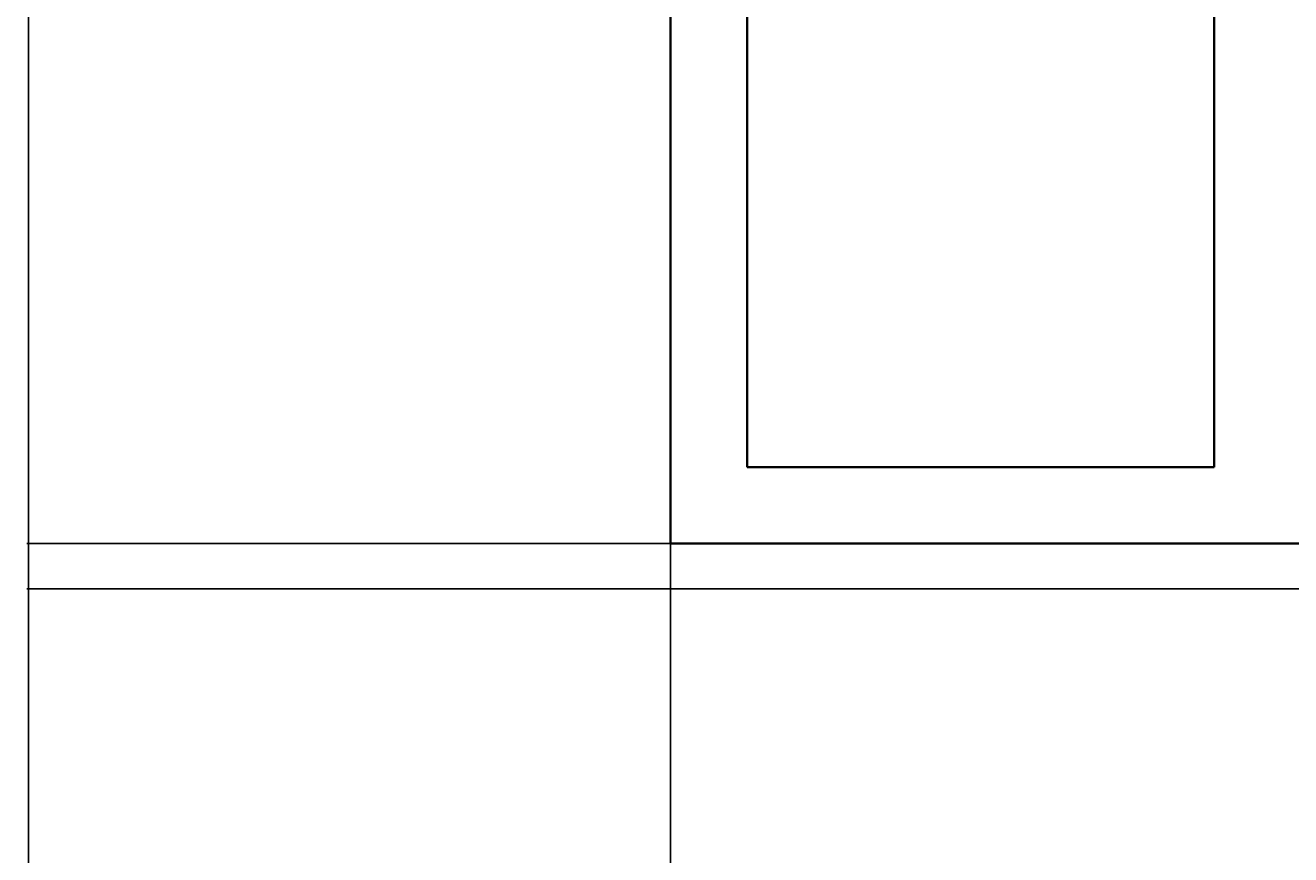
# Model space of a CAD drawing. Units: inches. Extents: x -61 to 1599, y -1316 to 257.
# Tile 43 of 204: x -61 to 88, y -478 to -380. Entities that reach past the tile are written whole.
import ezdxf

# ---------------------------------------------------------------- set-up
doc = ezdxf.new("R2010")
doc.units = ezdxf.units.IN
doc.header["$MEASUREMENT"] = 0
doc.layers.add('A-ANNO-DIMS', color=2, linetype='Continuous', lineweight=18)
doc.layers.add('WALLS', color=4, linetype='Continuous', lineweight=35)
doc.styles.get("Standard").update_dxf_attribs({"font": 'arial.ttf'})
doc.dimstyles.get("Standard").update_dxf_attribs({"dimtxt": 0.18, "dimasz": 0.18, "dimexe": 0.18, "dimexo": 0.0625, "dimgap": 0.09, "dimtad": 0, "dimtih": 1, "dimtoh": 1, "dimdec": 0, "dimzin": 0, "dimdsep": 46, "dimlunit": 3, "dimtxsty": 'Standard', "dimcen": 0.09, "dimadec": 0, "dimazin": 0, "dimtfac": 1, "dimtdec": 0, "dimtofl": 0, "dimtmove": 0, "dimatfit": 3, "dimfxl": 1, "dimtolj": 1, "dimtzin": 0, "dimarcsym": 0})

# ---------------------------------------------------------------- blocks, each defined once
blk = doc.blocks.new('*D687')
at = {"layer": 'A-ANNO-DIMS', "color": 0, "lineweight": -2, "transparency": 16777216}
for p, q in [((289.42, 181.68), (-61.08, 181.68)), ((-60.9, 181.5), (-60.9, -528.95)), ((-60.9, -1239.76), (-60.9, -529.32)), ((319.64, -1239.94), (-61.08, -1239.94))]:
    blk.add_line(p, q, dxfattribs=at)
at = {"layer": 'A-ANNO-DIMS', "color": 0, "transparency": 16777216}
for points in [[(-60.93, 181.5), (-60.87, 181.5), (-60.9, 181.68)], [(-60.93, -1239.76), (-60.87, -1239.76), (-60.9, -1239.94)]]:
    blk.add_solid(points, dxfattribs=at)
at = {"layer": 'DEFPOINTS', "color": 0, "transparency": 16777216}
for p in [(289.48, 181.68), (-60.9, -1239.94), (319.7, -1239.94)]:
    blk.add_point(p, dxfattribs=at)
at = {"layer": 'A-ANNO-DIMS', "color": 0, "transparency": 16777216, "insert": (-60.9, -529.13), "char_height": 0.18, "attachment_point": 5}
blk.add_mtext('\\A1;1421.6', dxfattribs=at)
blk = doc.blocks.new('*D691')
at = {"layer": 'A-ANNO-DIMS', "color": 0, "lineweight": -2, "transparency": 16777216}
for p, q in [((14.64, 157.68), (-61.08, 157.68)), ((-60.9, 157.5), (-60.9, -141.64)), ((-60.9, -441.14), (-60.9, -142)), ((14.64, -441.32), (-61.08, -441.32))]:
    blk.add_line(p, q, dxfattribs=at)
at = {"layer": 'A-ANNO-DIMS', "color": 0, "transparency": 16777216}
for points in [[(-60.93, 157.5), (-60.87, 157.5), (-60.9, 157.68)], [(-60.93, -441.14), (-60.87, -441.14), (-60.9, -441.32)]]:
    blk.add_solid(points, dxfattribs=at)
at = {"layer": 'DEFPOINTS', "color": 0, "transparency": 16777216}
for p in [(-60.9, 157.68), (14.7, 157.68), (14.7, -441.32)]:
    blk.add_point(p, dxfattribs=at)
at = {"layer": 'A-ANNO-DIMS', "color": 0, "transparency": 16777216, "insert": (-60.9, -141.82), "char_height": 0.18, "attachment_point": 5}
blk.add_mtext('\\A1;599', dxfattribs=at)
blk = doc.blocks.new('*D692')
at = {"layer": 'A-ANNO-DIMS', "color": 0, "lineweight": -2, "transparency": 16777216}
for p, q in [((14.64, -441.32), (-61.08, -441.32)), ((-60.9, -441.5), (-60.9, -528.95)), ((-60.9, -616.76), (-60.9, -529.32)), ((14.64, -616.94), (-61.08, -616.94))]:
    blk.add_line(p, q, dxfattribs=at)
at = {"layer": 'A-ANNO-DIMS', "color": 0, "transparency": 16777216}
for points in [[(-60.93, -441.5), (-60.87, -441.5), (-60.9, -441.32)], [(-60.93, -616.76), (-60.87, -616.76), (-60.9, -616.94)]]:
    blk.add_solid(points, dxfattribs=at)
at = {"layer": 'DEFPOINTS', "color": 0, "transparency": 16777216}
for p in [(-60.9, -441.32), (14.7, -441.32), (14.7, -616.94)]:
    blk.add_point(p, dxfattribs=at)
at = {"layer": 'A-ANNO-DIMS', "color": 0, "transparency": 16777216, "insert": (-60.9, -529.13), "char_height": 0.18, "attachment_point": 5}
blk.add_mtext('\\A1;175.62', dxfattribs=at)
blk = doc.blocks.new('*D699')
at = {"layer": 'A-ANNO-DIMS', "color": 0, "lineweight": -2, "transparency": 16777216}
for p, q in [((835.64, -167.17), (-61.08, -167.17)), ((-60.9, -167.35), (-60.9, -306.73)), ((-60.9, -446.47), (-60.9, -307.09)), ((841.64, -446.65), (-61.08, -446.65))]:
    blk.add_line(p, q, dxfattribs=at)
at = {"layer": 'A-ANNO-DIMS', "color": 0, "transparency": 16777216}
for points in [[(-60.93, -167.35), (-60.87, -167.35), (-60.9, -167.17)], [(-60.93, -446.47), (-60.87, -446.47), (-60.9, -446.65)]]:
    blk.add_solid(points, dxfattribs=at)
at = {"layer": 'DEFPOINTS', "color": 0, "transparency": 16777216}
for p in [(835.7, -167.17), (-60.9, -446.65), (841.7, -446.65)]:
    blk.add_point(p, dxfattribs=at)
at = {"layer": 'A-ANNO-DIMS', "color": 0, "transparency": 16777216, "insert": (-60.9, -306.91), "char_height": 0.18, "attachment_point": 5}
blk.add_mtext('\\A1;279.5', dxfattribs=at)
blk = doc.blocks.new('*D700')
at = {"layer": 'A-ANNO-DIMS', "color": 0, "lineweight": -2, "transparency": 16777216}
for p, q in [((14.7, -616.88), (14.7, 257.46)), ((14.88, 257.28), (96.77, 257.28)), ((179.57, 257.28), (97.68, 257.28)), ((179.75, -616.88), (179.75, 257.46))]:
    blk.add_line(p, q, dxfattribs=at)
at = {"layer": 'A-ANNO-DIMS', "color": 0, "transparency": 16777216}
for points in [[(14.88, 257.31), (14.88, 257.25), (14.7, 257.28)], [(179.57, 257.31), (179.57, 257.25), (179.75, 257.28)]]:
    blk.add_solid(points, dxfattribs=at)
at = {"layer": 'DEFPOINTS', "color": 0, "transparency": 16777216}
for p in [(179.75, 257.28), (14.7, -616.94), (179.75, -616.94)]:
    blk.add_point(p, dxfattribs=at)
at = {"layer": 'A-ANNO-DIMS', "color": 0, "transparency": 16777216, "insert": (97.23, 257.28), "char_height": 0.18, "attachment_point": 5}
blk.add_mtext('\\A1;165.05', dxfattribs=at)

msp = doc.modelspace()

# ---------------------------------------------------------------- linework, layer by layer
at = {"layer": 'WALLS'}
for p, q in [((14.7028, 157.6771), (14.7028, -441.3229)), ((23.7028, -175.3229), (23.7028, -432.3229)), ((78.7028, -175.3229), (78.7028, -432.3229)), ((23.7028, -432.3229), (78.7028, -432.3229)), ((14.7028, -441.3229), (237.7028, -441.3229))]:
    msp.add_line(p, q, dxfattribs=at)

# ---------------------------------------------------------------- dimensions: what is measured, and where the dimension line sits
at = {"layer": 'A-ANNO-DIMS'}
dim = msp.add_linear_dim(base=(179.7521, 257.2771), p1=(14.7028, -616.9446), p2=(179.7521, -616.9446), dimstyle='Standard', override={"dimdec": 2, "dimlfac": 1, "dimrnd": 0, "dimzin": 0, "dimdsep": 46, "dimlunit": 2}, dxfattribs=at)
dim.commit()
dim.dimension.update_dxf_attribs({"geometry": '*D700', "text_midpoint": (97.2274, 257.2771)})
for base, p1, p2, override, picture, middle in [((-60.8972, -1239.9446), (289.4807, 181.6771), (319.7028, -1239.9446), {"dimdec": 1, "dimlfac": 1, "dimrnd": 0, "dimzin": 0, "dimdsep": 46, "dimlunit": 2}, '*D687', (-60.8972, -529.1337)), ((-60.8972, 157.6771), (14.7028, -441.3229), (14.7028, 157.6771), {"dimdec": 0, "dimlfac": 1, "dimrnd": 0, "dimzin": 0, "dimdsep": 46, "dimlunit": 2}, '*D691', (-60.8972, -141.8229)), ((-60.8972, -446.6462), (835.7028, -167.169), (841.7028, -446.6462), {"dimdec": 1, "dimlfac": 1, "dimrnd": 0, "dimzin": 0, "dimdsep": 46, "dimlunit": 2}, '*D699', (-60.8972, -306.9076)), ((-60.8972, -441.3229), (14.7028, -616.9446), (14.7028, -441.3229), {"dimdec": 2, "dimlfac": 1, "dimrnd": 0, "dimzin": 0, "dimdsep": 46, "dimlunit": 2}, '*D692', (-60.8972, -529.1337))]:
    dim = msp.add_linear_dim(base=base, p1=p1, p2=p2, angle=90, dimstyle='Standard', override=override, dxfattribs=at)
    dim.commit()
    dim.dimension.update_dxf_attribs({"geometry": picture, "text_midpoint": middle})

doc.saveas('drawing.dxf')
